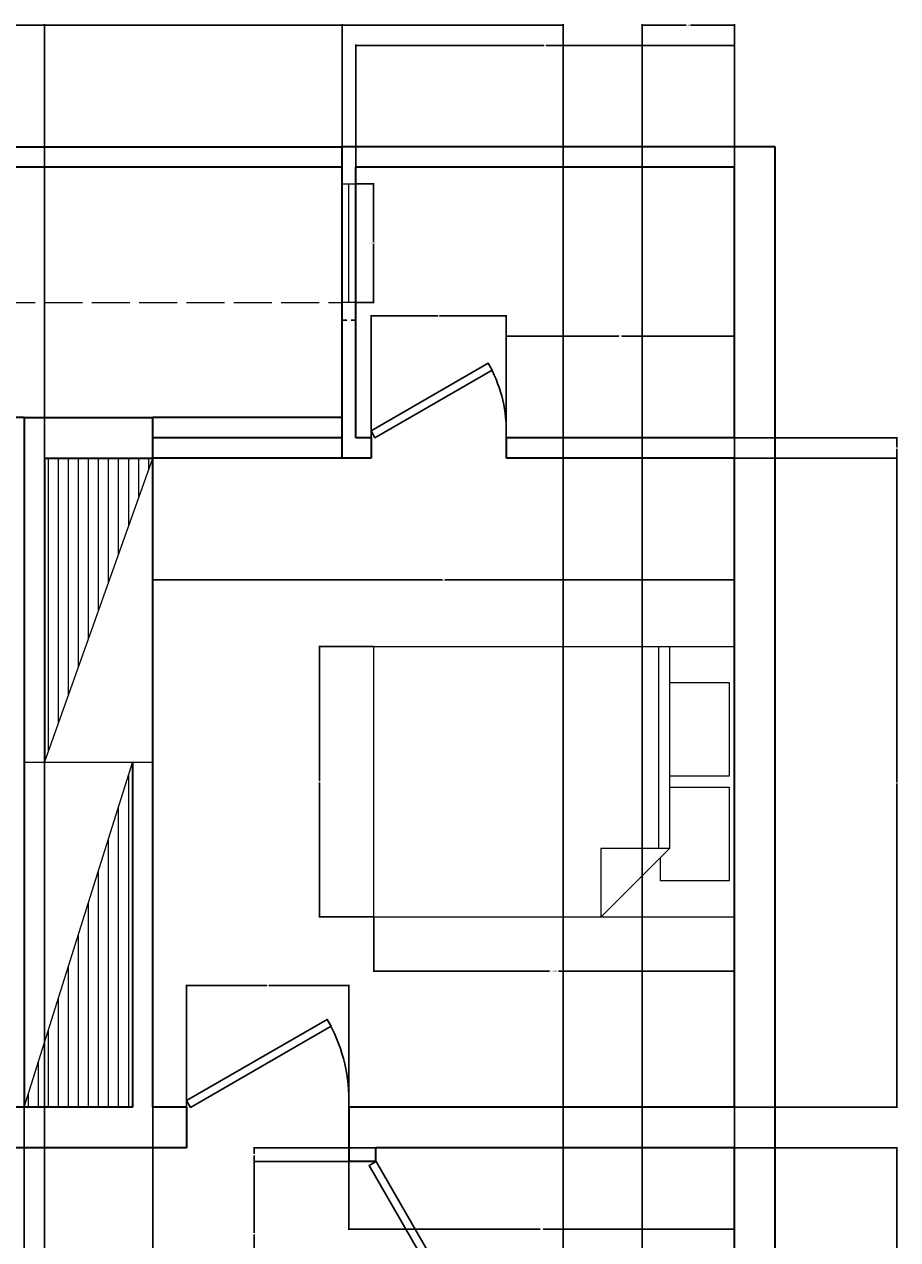
# Model space of a CAD drawing. Units: inches. Extents: x 2599 to 2953, y 557 to 1152.
# Tile 7 of 7: x 2759 to 2953, y 882 to 1152. Entities that reach past the tile are written whole.
import ezdxf

# ---------------------------------------------------------------- set-up
doc = ezdxf.new("R2010")
doc.units = ezdxf.units.IN
doc.linetypes.add('ACAD_ISO02W100', pattern=[15, 12, -3])
for name, color, linetype, lineweight in [('A-ANNO-DIMS', 2, 'Continuous', 18), ('A-DOOR', 4, 'Continuous', 25), ('A-FLOR-CABN', 9, 'Continuous', 18), ('A-FLOR-PATT', 252, 'Continuous', 13), ('A-FURN', 8, 'Continuous', 18), ('A-GLAZ', 4, 'Continuous', 18), ('A-WALL', 7, 'Continuous', 35), ('A-WALL-OVHD', 8, 'ACAD_ISO02W100', 18)]:
    doc.layers.add(name, color=color, linetype=linetype, lineweight=lineweight)
doc.styles.get("Standard").update_dxf_attribs({"font": 'arial.ttf'})
doc.dimstyles.get("Standard").update_dxf_attribs({"dimtxt": 0.18, "dimasz": 0.18, "dimexe": 0.18, "dimexo": 0.0625, "dimgap": 0.09, "dimtad": 0, "dimtih": 1, "dimtoh": 1, "dimdec": 4, "dimzin": 0, "dimdsep": 46, "dimtxsty": 'Standard', "dimcen": 0.09, "dimadec": 0, "dimazin": 0, "dimtfac": 1, "dimtdec": 4, "dimtofl": 0, "dimtmove": 0, "dimatfit": 3, "dimfxl": 1, "dimtolj": 1, "dimtzin": 0, "dimarcsym": 0})

# ---------------------------------------------------------------- blocks, each defined once
blk = doc.blocks.new('*U4')
for p, q in [((0, 0), (0, -6)), ((36, 0), (36, -6))]:
    blk.add_line(p, q)
blk.add_lwpolyline([(0, 0), (31.18, 18), (32.05, 16.48), (0.87, -1.52)], close=True)
blk.add_arc((0, 0), 36, 0, 30)
blk = doc.blocks.new('*U5')
for p, q in [((0, 0), (0, -6)), ((30, 0), (30, -6))]:
    blk.add_line(p, q)
blk.add_lwpolyline([(0, 0), (25.98, 15), (26.86, 13.48), (0.87, -1.52)], close=True)
blk.add_arc((0, 0), 30, 0, 30)
blk = doc.blocks.new('*U6')
for p, q in [((0, 0), (0, -6)), ((32, 0), (32, -6))]:
    blk.add_line(p, q)
blk.add_lwpolyline([(0, 0), (27.71, 16), (28.59, 14.48), (0.87, -1.52)], close=True)
blk.add_arc((0, 0), 32, 0, 30)
blk = doc.blocks.new('Bed - Queen')
for p, q in [((0, -80.00003), (0, 0)), ((0, 0), (59.99999, 0)), ((59.99999, 0), (59.99999, -80.00003)), ((7.99999, -1.2), (28.79998, -1.2)), ((7.99999, -14.4), (7.99999, -1.2)), ((28.79998, -1.2), (28.79998, -14.4)), ((31.19999, -1.2), (51.99999, -1.2)), ((31.19999, -14.4), (31.19999, -1.2)), ((51.99999, -1.2), (51.99999, -16.4)), ((0, -14.4), (44.8, -14.4)), ((59.99999, -29.6), (44.8, -14.4)), ((44.8, -14.4), (44.8, -29.6)), ((44.8, -16.8), (0, -16.8)), ((51.99999, -16.4), (46.79936, -16.4)), ((44.8, -29.6), (59.99999, -29.6)), ((59.99999, -80.00003), (0, -80.00003))]:
    blk.add_line(p, q)
blk = doc.blocks.new('WIN-26_335IN')
for p, q in [((0, 26.33), (3, 26.33)), ((1.5, 0), (1.5, 26.33)), ((3, 0), (0, 0))]:
    blk.add_line(p, q)
blk = doc.blocks.new('*D13')
at = {"layer": 'A-ANNO-DIMS', "color": 0, "lineweight": -2, "transparency": 16777216}
for p, q in [((2832.98, 1116.18), (2837.05, 1116.18)), ((2836.87, 1116), (2836.87, 1103.19)), ((2836.87, 1090.02), (2836.87, 1102.83)), ((2832.98, 1089.84), (2837.05, 1089.84))]:
    blk.add_line(p, q, dxfattribs=at)
at = {"layer": 'A-ANNO-DIMS', "color": 0, "transparency": 16777216}
for points in [[(2836.84, 1116), (2836.9, 1116), (2836.87, 1116.18)], [(2836.84, 1090.02), (2836.9, 1090.02), (2836.87, 1089.84)]]:
    blk.add_solid(points, dxfattribs=at)
at = {"layer": 'Defpoints', "color": 0, "transparency": 16777216}
for p in [(2832.92, 1116.18), (2836.87, 1116.18), (2832.92, 1089.84)]:
    blk.add_point(p, dxfattribs=at)
at = {"layer": 'A-ANNO-DIMS', "color": 0, "transparency": 16777216, "insert": (2836.87, 1103.01), "char_height": 0.18, "attachment_point": 5}
blk.add_mtext('\\A1;WINDOW 26 TYP.', dxfattribs=at)
blk = doc.blocks.new('*D14')
at = {"layer": 'A-ANNO-DIMS', "color": 0, "lineweight": -2, "transparency": 16777216}
for p, q in [((2829.92, 1089.78), (2829.92, 1085.71)), ((2832.92, 1089.78), (2832.92, 1085.71)), ((2830.1, 1085.89), (2830.96, 1085.89)), ((2832.74, 1085.89), (2831.88, 1085.89))]:
    blk.add_line(p, q, dxfattribs=at)
at = {"layer": 'A-ANNO-DIMS', "color": 0, "transparency": 16777216}
for points in [[(2830.1, 1085.92), (2830.1, 1085.86), (2829.92, 1085.89)], [(2832.74, 1085.92), (2832.74, 1085.86), (2832.92, 1085.89)]]:
    blk.add_solid(points, dxfattribs=at)
at = {"layer": 'Defpoints', "color": 0, "transparency": 16777216}
for p in [(2829.92, 1089.84), (2832.92, 1089.84), (2832.92, 1085.89)]:
    blk.add_point(p, dxfattribs=at)
at = {"layer": 'A-ANNO-DIMS', "color": 0, "transparency": 16777216, "insert": (2831.42, 1085.89), "char_height": 0.18, "attachment_point": 5}
blk.add_mtext('\\A1;3 TYP.', dxfattribs=at)
blk = doc.blocks.new('*D15')
at = {"layer": 'A-ANNO-DIMS', "color": 0, "lineweight": -2, "transparency": 16777216}
for p, q in [((2836.92, 953.48), (2836.92, 941.37)), ((2916.92, 953.48), (2916.92, 941.37)), ((2837.1, 941.55), (2875.93, 941.55)), ((2916.74, 941.55), (2877.92, 941.55))]:
    blk.add_line(p, q, dxfattribs=at)
at = {"layer": 'A-ANNO-DIMS', "color": 0, "transparency": 16777216}
for points in [[(2837.1, 941.58), (2837.1, 941.52), (2836.92, 941.55)], [(2916.74, 941.58), (2916.74, 941.52), (2916.92, 941.55)]]:
    blk.add_solid(points, dxfattribs=at)
at = {"layer": 'Defpoints', "color": 0, "transparency": 16777216}
for p in [(2836.92, 953.55), (2916.92, 953.55), (2916.92, 941.55)]:
    blk.add_point(p, dxfattribs=at)
at = {"layer": 'A-ANNO-DIMS', "color": 0, "transparency": 16777216, "insert": (2876.92, 941.55), "char_height": 0.18, "attachment_point": 5}
blk.add_mtext('\\A1;QUEEN BED 80', dxfattribs=at)
blk = doc.blocks.new('*D16')
at = {"layer": 'A-ANNO-DIMS', "color": 0, "lineweight": -2, "transparency": 16777216}
for p, q in [((2836.86, 1013.55), (2824.74, 1013.55)), ((2824.92, 1013.37), (2824.92, 983.73)), ((2824.92, 953.73), (2824.92, 983.36)), ((2836.86, 953.55), (2824.74, 953.55))]:
    blk.add_line(p, q, dxfattribs=at)
at = {"layer": 'A-ANNO-DIMS', "color": 0, "transparency": 16777216}
for points in [[(2824.89, 1013.37), (2824.95, 1013.37), (2824.92, 1013.55)], [(2824.89, 953.73), (2824.95, 953.73), (2824.92, 953.55)]]:
    blk.add_solid(points, dxfattribs=at)
at = {"layer": 'Defpoints', "color": 0, "transparency": 16777216}
for p in [(2836.92, 1013.55), (2824.92, 953.55), (2836.92, 953.55)]:
    blk.add_point(p, dxfattribs=at)
at = {"layer": 'A-ANNO-DIMS', "color": 0, "transparency": 16777216, "insert": (2824.92, 983.55), "char_height": 0.18, "attachment_point": 5}
blk.add_mtext('\\A1;60', dxfattribs=at)
blk = doc.blocks.new('*D21')
at = {"layer": 'A-ANNO-DIMS', "color": 0, "lineweight": -2, "transparency": 16777216}
for p, q in [((2625.92, 1124.28), (2625.92, 557.16)), ((2925.92, 584.28), (2925.92, 557.16)), ((2626.1, 557.34), (2775.63, 557.34)), ((2925.74, 557.34), (2776.21, 557.34))]:
    blk.add_line(p, q, dxfattribs=at)
at = {"layer": 'A-ANNO-DIMS', "color": 0, "transparency": 16777216}
for points in [[(2626.1, 557.37), (2626.1, 557.31), (2625.92, 557.34)], [(2925.74, 557.37), (2925.74, 557.31), (2925.92, 557.34)]]:
    blk.add_solid(points, dxfattribs=at)
at = {"layer": 'Defpoints', "color": 0, "transparency": 16777216}
for p in [(2625.92, 1124.34), (2925.92, 584.34), (2925.92, 557.34)]:
    blk.add_point(p, dxfattribs=at)
at = {"layer": 'A-ANNO-DIMS', "color": 0, "transparency": 16777216, "insert": (2775.92, 557.34), "char_height": 0.18, "attachment_point": 5}
blk.add_mtext('\\A1;300', dxfattribs=at)
blk = doc.blocks.new('*D25')
at = {"layer": 'A-ANNO-DIMS', "color": 0, "lineweight": -2, "transparency": 16777216}
for p, q in [((2916.98, 902.34), (2953.1, 902.34)), ((2952.92, 902.16), (2952.92, 836.52)), ((2952.92, 770.52), (2952.92, 836.16)), ((2916.98, 770.34), (2953.1, 770.34))]:
    blk.add_line(p, q, dxfattribs=at)
at = {"layer": 'A-ANNO-DIMS', "color": 0, "transparency": 16777216}
for points in [[(2952.89, 902.16), (2952.95, 902.16), (2952.92, 902.34)], [(2952.89, 770.52), (2952.95, 770.52), (2952.92, 770.34)]]:
    blk.add_solid(points, dxfattribs=at)
at = {"layer": 'Defpoints', "color": 0, "transparency": 16777216}
for p in [(2916.92, 902.34), (2952.92, 902.34), (2916.92, 770.34)]:
    blk.add_point(p, dxfattribs=at)
at = {"layer": 'A-ANNO-DIMS', "color": 0, "transparency": 16777216, "insert": (2952.92, 836.34), "char_height": 0.18, "attachment_point": 5}
blk.add_mtext('\\A1;132', dxfattribs=at)
blk = doc.blocks.new('*D26')
at = {"layer": 'A-ANNO-DIMS', "color": 0, "lineweight": -2, "transparency": 16777216}
for p, q in [((2837.36, 899.34), (2810.24, 899.34)), ((2810.42, 899.16), (2810.42, 883.52)), ((2810.42, 867.52), (2810.42, 883.16)), ((2837.36, 867.34), (2810.24, 867.34))]:
    blk.add_line(p, q, dxfattribs=at)
at = {"layer": 'A-ANNO-DIMS', "color": 0, "transparency": 16777216}
for points in [[(2810.39, 899.16), (2810.45, 899.16), (2810.42, 899.34)], [(2810.39, 867.52), (2810.45, 867.52), (2810.42, 867.34)]]:
    blk.add_solid(points, dxfattribs=at)
at = {"layer": 'Defpoints', "color": 0, "transparency": 16777216}
for p in [(2810.42, 899.34), (2837.42, 899.34), (2837.42, 867.34)]:
    blk.add_point(p, dxfattribs=at)
at = {"layer": 'A-ANNO-DIMS', "color": 0, "transparency": 16777216, "insert": (2810.42, 883.34), "char_height": 0.18, "attachment_point": 5}
blk.add_mtext('\\A1;32', dxfattribs=at)
blk = doc.blocks.new('*D27')
at = {"layer": 'A-ANNO-DIMS', "color": 0, "lineweight": -2, "transparency": 16777216}
for p, q in [((2837.36, 902.34), (2810.24, 902.34)), ((2810.42, 902.16), (2810.42, 901.02)), ((2810.42, 899.52), (2810.42, 900.66)), ((2837.36, 899.34), (2810.24, 899.34))]:
    blk.add_line(p, q, dxfattribs=at)
at = {"layer": 'A-ANNO-DIMS', "color": 0, "transparency": 16777216}
for points in [[(2810.39, 902.16), (2810.45, 902.16), (2810.42, 902.34)], [(2810.39, 899.52), (2810.45, 899.52), (2810.42, 899.34)]]:
    blk.add_solid(points, dxfattribs=at)
at = {"layer": 'Defpoints', "color": 0, "transparency": 16777216}
for p in [(2810.42, 902.34), (2837.42, 902.34), (2837.42, 899.34)]:
    blk.add_point(p, dxfattribs=at)
at = {"layer": 'A-ANNO-DIMS', "color": 0, "transparency": 16777216, "insert": (2810.42, 900.84), "char_height": 0.18, "attachment_point": 5}
blk.add_mtext('\\A1;3', dxfattribs=at)
blk = doc.blocks.new('*D38')
at = {"layer": 'A-ANNO-DIMS', "color": 0, "lineweight": -2, "transparency": 16777216}
for p, q in [((2763.92, 761.4), (2763.92, 1151.53)), ((2764.1, 1151.35), (2821.14, 1151.35)), ((2878.74, 1151.35), (2821.7, 1151.35)), ((2878.92, 761.4), (2878.92, 1151.53))]:
    blk.add_line(p, q, dxfattribs=at)
at = {"layer": 'A-ANNO-DIMS', "color": 0, "transparency": 16777216}
for points in [[(2764.1, 1151.38), (2764.1, 1151.32), (2763.92, 1151.35)], [(2878.74, 1151.38), (2878.74, 1151.32), (2878.92, 1151.35)]]:
    blk.add_solid(points, dxfattribs=at)
at = {"layer": 'Defpoints', "color": 0, "transparency": 16777216}
for p in [(2878.92, 1151.35), (2763.92, 761.34), (2878.92, 761.34)]:
    blk.add_point(p, dxfattribs=at)
at = {"layer": 'A-ANNO-DIMS', "color": 0, "transparency": 16777216, "insert": (2821.42, 1151.35), "char_height": 0.18, "attachment_point": 5}
blk.add_mtext('\\A1;115', dxfattribs=at)
blk = doc.blocks.new('*D39')
at = {"layer": 'A-ANNO-DIMS', "color": 0, "lineweight": -2, "transparency": 16777216}
for p, q in [((2896.44, 761.4), (2896.44, 1151.53)), ((2896.62, 1151.35), (2906.21, 1151.35)), ((2916.74, 1151.35), (2907.14, 1151.35)), ((2916.92, 761.4), (2916.92, 1151.53))]:
    blk.add_line(p, q, dxfattribs=at)
at = {"layer": 'A-ANNO-DIMS', "color": 0, "transparency": 16777216}
for points in [[(2896.62, 1151.38), (2896.62, 1151.32), (2896.44, 1151.35)], [(2916.74, 1151.38), (2916.74, 1151.32), (2916.92, 1151.35)]]:
    blk.add_solid(points, dxfattribs=at)
at = {"layer": 'Defpoints', "color": 0, "transparency": 16777216}
for p in [(2916.92, 1151.35), (2896.44, 761.34), (2916.92, 761.34)]:
    blk.add_point(p, dxfattribs=at)
at = {"layer": 'A-ANNO-DIMS', "color": 0, "transparency": 16777216, "insert": (2906.68, 1151.35), "char_height": 0.18, "attachment_point": 5}
blk.add_mtext('\\A1;20.483', dxfattribs=at)
blk = doc.blocks.new('*D55')
at = {"layer": 'A-ANNO-DIMS', "color": 0, "lineweight": -2, "transparency": 16777216}
for p, q in [((2759.42, 911.28), (2759.42, 557.16)), ((2787.92, 911.28), (2787.92, 557.16)), ((2759.6, 557.34), (2773.35, 557.34)), ((2787.74, 557.34), (2774, 557.34))]:
    blk.add_line(p, q, dxfattribs=at)
at = {"layer": 'A-ANNO-DIMS', "color": 0, "transparency": 16777216}
for points in [[(2759.6, 557.37), (2759.6, 557.31), (2759.42, 557.34)], [(2787.74, 557.37), (2787.74, 557.31), (2787.92, 557.34)]]:
    blk.add_solid(points, dxfattribs=at)
at = {"layer": 'Defpoints', "color": 0, "transparency": 16777216}
for p in [(2759.42, 911.34), (2787.92, 911.34), (2787.92, 557.34)]:
    blk.add_point(p, dxfattribs=at)
at = {"layer": 'A-ANNO-DIMS', "color": 0, "transparency": 16777216, "insert": (2773.67, 557.34), "char_height": 0.18, "attachment_point": 5}
blk.add_mtext('\\A1;28.5', dxfattribs=at)
blk = doc.blocks.new('*D56')
at = {"layer": 'A-ANNO-DIMS', "color": 0, "lineweight": -2, "transparency": 16777216}
for p, q in [((2787.92, 1055.28), (2787.92, 1028.16)), ((2916.92, 1055.28), (2916.92, 1028.16)), ((2788.1, 1028.34), (2852.14, 1028.34)), ((2916.74, 1028.34), (2852.7, 1028.34))]:
    blk.add_line(p, q, dxfattribs=at)
at = {"layer": 'A-ANNO-DIMS', "color": 0, "transparency": 16777216}
for points in [[(2788.1, 1028.37), (2788.1, 1028.31), (2787.92, 1028.34)], [(2916.74, 1028.37), (2916.74, 1028.31), (2916.92, 1028.34)]]:
    blk.add_solid(points, dxfattribs=at)
at = {"layer": 'Defpoints', "color": 0, "transparency": 16777216}
for p in [(2787.92, 1055.34), (2916.92, 1055.34), (2787.92, 1028.34)]:
    blk.add_point(p, dxfattribs=at)
at = {"layer": 'A-ANNO-DIMS', "color": 0, "transparency": 16777216, "insert": (2852.42, 1028.34), "char_height": 0.18, "attachment_point": 5}
blk.add_mtext('\\A1;129', dxfattribs=at)
blk = doc.blocks.new('*D57')
at = {"layer": 'A-ANNO-DIMS', "color": 0, "lineweight": -2, "transparency": 16777216}
for p, q in [((2916.98, 1055.34), (2953.1, 1055.34)), ((2952.92, 1055.16), (2952.92, 983.52)), ((2952.92, 911.52), (2952.92, 983.16)), ((2916.98, 911.34), (2953.1, 911.34))]:
    blk.add_line(p, q, dxfattribs=at)
at = {"layer": 'A-ANNO-DIMS', "color": 0, "transparency": 16777216}
for points in [[(2952.89, 1055.16), (2952.95, 1055.16), (2952.92, 1055.34)], [(2952.89, 911.52), (2952.95, 911.52), (2952.92, 911.34)]]:
    blk.add_solid(points, dxfattribs=at)
at = {"layer": 'Defpoints', "color": 0, "transparency": 16777216}
for p in [(2916.92, 1055.34), (2952.92, 1055.34), (2916.92, 911.34)]:
    blk.add_point(p, dxfattribs=at)
at = {"layer": 'A-ANNO-DIMS', "color": 0, "transparency": 16777216, "insert": (2952.92, 983.34), "char_height": 0.18, "attachment_point": 5}
blk.add_mtext('\\A1;144', dxfattribs=at)
blk = doc.blocks.new('*D59')
at = {"layer": 'A-ANNO-DIMS', "color": 0, "lineweight": -2, "transparency": 16777216}
for p, q in [((2721.92, 1124.4), (2721.92, 1151.53)), ((2722.1, 1151.35), (2775.64, 1151.35)), ((2829.74, 1151.35), (2776.2, 1151.35)), ((2829.92, 1124.4), (2829.92, 1151.53))]:
    blk.add_line(p, q, dxfattribs=at)
at = {"layer": 'A-ANNO-DIMS', "color": 0, "transparency": 16777216}
for points in [[(2722.1, 1151.38), (2722.1, 1151.32), (2721.92, 1151.35)], [(2829.74, 1151.38), (2829.74, 1151.32), (2829.92, 1151.35)]]:
    blk.add_solid(points, dxfattribs=at)
at = {"layer": 'Defpoints', "color": 0, "transparency": 16777216}
for p in [(2829.92, 1151.35), (2721.92, 1124.34), (2829.92, 1124.34)]:
    blk.add_point(p, dxfattribs=at)
at = {"layer": 'A-ANNO-DIMS', "color": 0, "transparency": 16777216, "insert": (2775.92, 1151.35), "char_height": 0.18, "attachment_point": 5}
blk.add_mtext('\\A1;108', dxfattribs=at)
blk = doc.blocks.new('*D60')
at = {"layer": 'A-ANNO-DIMS', "color": 0, "lineweight": -2, "transparency": 16777216}
for p, q in [((2832.92, 1119.9), (2832.92, 1147.03)), ((2833.1, 1146.85), (2874.7, 1146.85)), ((2916.74, 1146.85), (2875.14, 1146.85)), ((2916.92, 1119.9), (2916.92, 1147.03))]:
    blk.add_line(p, q, dxfattribs=at)
at = {"layer": 'A-ANNO-DIMS', "color": 0, "transparency": 16777216}
for points in [[(2833.1, 1146.88), (2833.1, 1146.82), (2832.92, 1146.85)], [(2916.74, 1146.88), (2916.74, 1146.82), (2916.92, 1146.85)]]:
    blk.add_solid(points, dxfattribs=at)
at = {"layer": 'Defpoints', "color": 0, "transparency": 16777216}
for p in [(2916.92, 1146.85), (2832.92, 1119.84), (2916.92, 1119.84)]:
    blk.add_point(p, dxfattribs=at)
at = {"layer": 'A-ANNO-DIMS', "color": 0, "transparency": 16777216, "insert": (2874.92, 1146.85), "char_height": 0.18, "attachment_point": 5}
blk.add_mtext('\\A1;84', dxfattribs=at)
blk = doc.blocks.new('*D64')
at = {"layer": 'A-ANNO-DIMS', "color": 0, "lineweight": -2, "transparency": 16777216}
for p, q in [((2836.32, 1059.9), (2836.32, 1087.03)), ((2836.5, 1086.85), (2851.1, 1086.85)), ((2866.14, 1086.85), (2851.54, 1086.85)), ((2866.32, 1059.9), (2866.32, 1087.03))]:
    blk.add_line(p, q, dxfattribs=at)
at = {"layer": 'A-ANNO-DIMS', "color": 0, "transparency": 16777216}
for points in [[(2836.5, 1086.88), (2836.5, 1086.82), (2836.32, 1086.85)], [(2866.14, 1086.88), (2866.14, 1086.82), (2866.32, 1086.85)]]:
    blk.add_solid(points, dxfattribs=at)
at = {"layer": 'Defpoints', "color": 0, "transparency": 16777216}
for p in [(2866.32, 1086.85), (2836.32, 1059.84), (2866.32, 1059.84)]:
    blk.add_point(p, dxfattribs=at)
at = {"layer": 'A-ANNO-DIMS', "color": 0, "transparency": 16777216, "insert": (2851.32, 1086.85), "char_height": 0.18, "attachment_point": 5}
blk.add_mtext('\\A1;30', dxfattribs=at)
blk = doc.blocks.new('*D65')
at = {"layer": 'A-ANNO-DIMS', "color": 0, "lineweight": -2, "transparency": 16777216}
for p, q in [((2866.32, 1055.4), (2866.32, 1082.53)), ((2866.5, 1082.35), (2891.3, 1082.35)), ((2916.74, 1082.35), (2891.94, 1082.35)), ((2916.92, 1055.4), (2916.92, 1082.53))]:
    blk.add_line(p, q, dxfattribs=at)
at = {"layer": 'A-ANNO-DIMS', "color": 0, "transparency": 16777216}
for points in [[(2866.5, 1082.38), (2866.5, 1082.32), (2866.32, 1082.35)], [(2916.74, 1082.38), (2916.74, 1082.32), (2916.92, 1082.35)]]:
    blk.add_solid(points, dxfattribs=at)
at = {"layer": 'Defpoints', "color": 0, "transparency": 16777216}
for p in [(2916.92, 1082.35), (2866.32, 1055.34), (2916.92, 1055.34)]:
    blk.add_point(p, dxfattribs=at)
at = {"layer": 'A-ANNO-DIMS', "color": 0, "transparency": 16777216, "insert": (2891.62, 1082.35), "char_height": 0.18, "attachment_point": 5}
blk.add_mtext('\\A1;50.6', dxfattribs=at)
blk = doc.blocks.new('*D68')
at = {"layer": 'A-ANNO-DIMS', "color": 0, "lineweight": -2, "transparency": 16777216}
for p, q in [((2795.42, 911.4), (2795.42, 938.53)), ((2795.6, 938.35), (2813.21, 938.35)), ((2831.24, 938.35), (2813.64, 938.35)), ((2831.42, 911.4), (2831.42, 938.53))]:
    blk.add_line(p, q, dxfattribs=at)
at = {"layer": 'A-ANNO-DIMS', "color": 0, "transparency": 16777216}
for points in [[(2795.6, 938.38), (2795.6, 938.32), (2795.42, 938.35)], [(2831.24, 938.38), (2831.24, 938.32), (2831.42, 938.35)]]:
    blk.add_solid(points, dxfattribs=at)
at = {"layer": 'Defpoints', "color": 0, "transparency": 16777216}
for p in [(2831.42, 938.35), (2795.42, 911.34), (2831.42, 911.34)]:
    blk.add_point(p, dxfattribs=at)
at = {"layer": 'A-ANNO-DIMS', "color": 0, "transparency": 16777216, "insert": (2813.42, 938.35), "char_height": 0.18, "attachment_point": 5}
blk.add_mtext('\\A1;36', dxfattribs=at)
blk = doc.blocks.new('*D69')
at = {"layer": 'A-ANNO-DIMS', "color": 0, "lineweight": -2, "transparency": 16777216}
for p, q in [((2831.42, 911.28), (2831.42, 884.16)), ((2916.92, 911.28), (2916.92, 884.16)), ((2831.6, 884.34), (2873.85, 884.34)), ((2916.74, 884.34), (2874.5, 884.34))]:
    blk.add_line(p, q, dxfattribs=at)
at = {"layer": 'A-ANNO-DIMS', "color": 0, "transparency": 16777216}
for points in [[(2831.6, 884.37), (2831.6, 884.31), (2831.42, 884.34)], [(2916.74, 884.37), (2916.74, 884.31), (2916.92, 884.34)]]:
    blk.add_solid(points, dxfattribs=at)
at = {"layer": 'Defpoints', "color": 0, "transparency": 16777216}
for p in [(2831.42, 911.34), (2916.92, 911.34), (2831.42, 884.34)]:
    blk.add_point(p, dxfattribs=at)
at = {"layer": 'A-ANNO-DIMS', "color": 0, "transparency": 16777216, "insert": (2874.17, 884.34), "char_height": 0.18, "attachment_point": 5}
blk.add_mtext('\\A1;85.5', dxfattribs=at)
blk = doc.blocks.new('*D71')
at = {"layer": 'A-ANNO-DIMS', "color": 0, "lineweight": -2, "transparency": 16777216}
for p, q in [((2829.86, 1119.84), (2598.74, 1119.84)), ((2598.92, 1119.66), (2598.92, 1092.27)), ((2598.92, 1064.52), (2598.92, 1091.91)), ((2787.86, 1064.34), (2598.74, 1064.34))]:
    blk.add_line(p, q, dxfattribs=at)
at = {"layer": 'A-ANNO-DIMS', "color": 0, "transparency": 16777216}
for points in [[(2598.89, 1119.66), (2598.95, 1119.66), (2598.92, 1119.84)], [(2598.89, 1064.52), (2598.95, 1064.52), (2598.92, 1064.34)]]:
    blk.add_solid(points, dxfattribs=at)
at = {"layer": 'Defpoints', "color": 0, "transparency": 16777216}
for p in [(2598.92, 1119.84), (2829.92, 1119.84), (2787.92, 1064.34)]:
    blk.add_point(p, dxfattribs=at)
at = {"layer": 'A-ANNO-DIMS', "color": 0, "transparency": 16777216, "insert": (2598.92, 1092.09), "char_height": 0.18, "attachment_point": 5}
blk.add_mtext('\\A1;55.5', dxfattribs=at)
blk = doc.blocks.new('*D73')
at = {"layer": 'A-ANNO-DIMS', "color": 0, "lineweight": -2, "transparency": 16777216}
for p, q in [((2916.98, 1059.84), (2953.1, 1059.84)), ((2952.92, 1059.66), (2952.92, 1057.77)), ((2952.92, 1055.52), (2952.92, 1057.41)), ((2916.98, 1055.34), (2953.1, 1055.34))]:
    blk.add_line(p, q, dxfattribs=at)
at = {"layer": 'A-ANNO-DIMS', "color": 0, "transparency": 16777216}
for points in [[(2952.89, 1059.66), (2952.95, 1059.66), (2952.92, 1059.84)], [(2952.89, 1055.52), (2952.95, 1055.52), (2952.92, 1055.34)]]:
    blk.add_solid(points, dxfattribs=at)
at = {"layer": 'Defpoints', "color": 0, "transparency": 16777216}
for p in [(2916.92, 1059.84), (2952.92, 1059.84), (2916.92, 1055.34)]:
    blk.add_point(p, dxfattribs=at)
at = {"layer": 'A-ANNO-DIMS', "color": 0, "transparency": 16777216, "insert": (2952.92, 1057.59), "char_height": 0.18, "attachment_point": 5}
blk.add_mtext('\\A1;4.5', dxfattribs=at)

msp = doc.modelspace()

# ---------------------------------------------------------------- hatches: boundary and pattern name
at = {"layer": 'A-FLOR-PATT'}
h = msp.add_hatch(dxfattribs=at)
h.set_pattern_fill('ANSI31', color=256, scale=0.7, angle=45)
h.paths.add_polyline_path([(2763.9211, 987.8417), (2787.9211, 1055.3417), (2763.9211, 1055.3417)])
h.paths.add_polyline_path([(2783.4211, 987.8417), (2759.4211, 911.3417), (2783.4211, 911.3417)])

# ---------------------------------------------------------------- linework, layer by layer
at = {"layer": 'A-FLOR-CABN'}
for p, q in [((2763.9211, 987.8417), (2787.9211, 1055.3417)), ((2787.9211, 987.8417), (2759.4211, 987.8417)), ((2759.4211, 911.3417), (2783.4211, 987.8417))]:
    msp.add_line(p, q, dxfattribs=at)
at = {"layer": 'A-WALL'}
for p, q in [((2721.9211, 1124.3417), (2829.9211, 1124.3417)), ((2925.9211, 1124.3417), (2829.9211, 1124.3417)), ((2829.9211, 1055.3417), (2829.9211, 1124.3417)), ((2925.9211, 584.3417), (2925.9211, 1124.3417)), ((2829.9211, 1119.8417), (2721.9211, 1119.8417)), ((2916.9211, 1119.8417), (2832.9211, 1119.8417)), ((2832.9211, 1059.8417), (2832.9211, 1119.8417)), ((2916.9211, 1059.8417), (2916.9211, 1119.8417)), ((2759.4211, 1064.3417), (2721.9211, 1064.3417)), ((2759.4211, 1064.3417), (2759.4211, 911.3417)), ((2759.4211, 1064.3417), (2787.9211, 1064.3417)), ((2787.9211, 911.3417), (2787.9211, 1064.3417)), ((2829.9211, 1064.3417), (2787.9211, 1064.3417)), ((2829.9211, 1059.8417), (2787.9211, 1059.8417)), ((2836.3211, 1059.8417), (2832.9211, 1059.8417)), ((2836.3211, 1059.8417), (2836.3211, 1055.3417)), ((2916.9211, 1059.8417), (2866.3211, 1059.8417)), ((2866.3211, 1059.8417), (2866.3211, 1055.3417)), ((2763.9211, 1055.3417), (2763.9211, 987.8417)), ((2763.9211, 1055.3417), (2787.9211, 1055.3417)), ((2829.9211, 1055.3417), (2787.9211, 1055.3417)), ((2836.3211, 1055.3417), (2829.9211, 1055.3417)), ((2916.9211, 1055.3417), (2866.3211, 1055.3417)), ((2916.9211, 911.3417), (2916.9211, 1055.3417)), ((2783.4211, 987.8417), (2783.4211, 911.3417)), ((2783.4211, 911.3417), (2753.3499, 911.3417)), ((2795.4243, 911.3417), (2787.9211, 911.3417)), ((2795.4243, 911.3417), (2795.4243, 902.3417)), ((2916.9211, 911.3417), (2831.4243, 911.3417)), ((2831.4243, 911.3417), (2831.4243, 899.3417)), ((2795.4243, 902.3417), (2753.3499, 902.3417)), ((2831.4243, 902.3417), (2831.4211, 902.3417)), ((2916.9211, 902.3417), (2837.4211, 902.3417)), ((2837.4211, 899.3417), (2837.4211, 902.3417)), ((2916.9211, 770.3417), (2916.9211, 902.3417)), ((2837.4211, 899.3417), (2831.4243, 899.3417))]:
    msp.add_line(p, q, dxfattribs=at)
at = {"layer": 'A-WALL-OVHD', "ltscale": 0.7}
msp.add_line((2721.9211, 1089.8417), (2829.9211, 1089.8417), dxfattribs=at)

# ---------------------------------------------------------------- block references
at = {"layer": 'A-DOOR'}
for name, p in [('*U5', (2836.3211, 1061.3417)), ('*U4', (2795.4243, 912.8417))]:
    msp.add_blockref(name, p, dxfattribs=at)
at = {"layer": 'A-DOOR', "rotation": 270}
msp.add_blockref('*U6', (2837.4243, 899.3417), dxfattribs=at)
at = {"layer": 'A-FURN', "rotation": 270}
msp.add_blockref('Bed - Queen', (2916.9211, 1013.5463), dxfattribs=at)
at = {"layer": 'A-GLAZ'}
msp.add_blockref('WIN-26_335IN', (2829.921, 1089.842), dxfattribs=at)

# ---------------------------------------------------------------- dimensions: what is measured, and where the dimension line sits
at = {"layer": 'A-ANNO-DIMS'}
for base, p1, p2, override, picture, middle in [((2829.9211, 1151.3452), (2721.9211, 1124.3417), (2829.9211, 1124.3417), {"dimdec": 0, "dimlfac": 1, "dimrnd": 0, "dimzin": 0, "dimdsep": 46, "dimlunit": 2}, '*D59', (2775.9211, 1151.3452)), ((2878.9211, 1151.3452), (2763.9211, 761.3417), (2878.9211, 761.3417), {"dimdec": 0, "dimlfac": 1, "dimrnd": 0, "dimzin": 0, "dimdsep": 46, "dimlunit": 2}, '*D38', (2821.4211, 1151.3452)), ((2916.92111, 1151.34517), (2896.43762, 761.34167), (2916.92111, 761.34167), {"dimdec": 3, "dimlfac": 1, "dimrnd": 0, "dimzin": 0, "dimdsep": 46, "dimlunit": 2}, '*D39', (2906.67936, 1151.34517)), ((2916.9211, 1146.8452), (2832.9211, 1119.8417), (2916.9211, 1119.8417), {"dimdec": 0, "dimlfac": 1, "dimrnd": 0, "dimzin": 0, "dimdsep": 46, "dimlunit": 2}, '*D60', (2874.9211, 1146.8452)), ((2925.9211, 557.3382), (2625.9211, 1124.3417), (2925.9211, 584.3417), {"dimdec": 0, "dimlfac": 1, "dimrnd": 0, "dimzin": 0, "dimdsep": 46, "dimlunit": 2}, '*D21', (2775.9211, 557.3382)), ((2866.3211, 1086.8452), (2836.3211, 1059.8417), (2866.3211, 1059.8417), {"dimdec": 0, "dimlfac": 1, "dimrnd": 0, "dimzin": 0, "dimdsep": 46, "dimlunit": 2}, '*D64', (2851.3211, 1086.8452)), ((2916.9211, 1082.3452), (2866.3211, 1055.3417), (2916.9211, 1055.3417), {"dimdec": 1, "dimlfac": 1, "dimrnd": 0, "dimzin": 0, "dimdsep": 46, "dimlunit": 2}, '*D65', (2891.6211, 1082.3452)), ((2831.4243, 938.3452), (2795.4243, 911.3417), (2831.4243, 911.3417), {"dimdec": 0, "dimlfac": 1, "dimrnd": 0, "dimzin": 0, "dimdsep": 46, "dimlunit": 2}, '*D68', (2813.4243, 938.3452)), ((2787.9211, 557.3382), (2759.4211, 911.3417), (2787.9211, 911.3417), {"dimdec": 1, "dimlfac": 1, "dimrnd": 0, "dimzin": 0, "dimdsep": 46, "dimlunit": 2}, '*D55', (2773.6711, 557.3382))]:
    dim = msp.add_linear_dim(base=base, p1=p1, p2=p2, dimstyle='Standard', override=override, dxfattribs=at)
    dim.commit()
    dim.dimension.update_dxf_attribs({"geometry": picture, "text_midpoint": middle})
for base, p1, p2, angle, override, picture, middle in [((2598.9176, 1119.8417), (2787.9211, 1064.3417), (2829.9211, 1119.8417), 90, {"dimdec": 1, "dimlfac": 1, "dimrnd": 0, "dimzin": 0, "dimdsep": 46, "dimlunit": 2}, '*D71', (2598.9176, 1092.0917)), ((2952.9246, 1059.8417), (2916.9211, 1055.3417), (2916.9211, 1059.8417), 90, {"dimdec": 1, "dimlfac": 1, "dimrnd": 0, "dimzin": 0, "dimdsep": 46, "dimlunit": 2}, '*D73', (2952.9246, 1057.5917)), ((2787.9211, 1028.3382), (2916.9211, 1055.3417), (2787.9211, 1055.3417), 180, {"dimdec": 0, "dimlfac": 1, "dimrnd": 0, "dimzin": 0, "dimdsep": 46, "dimlunit": 2}, '*D56', (2852.4211, 1028.3382)), ((2952.9246, 1055.3417), (2916.9211, 911.3417), (2916.9211, 1055.3417), 90, {"dimdec": 0, "dimlfac": 1, "dimrnd": 0, "dimzin": 0, "dimdsep": 46, "dimlunit": 2}, '*D57', (2952.9246, 983.3417)), ((2824.9211, 953.5463), (2836.9211, 1013.5463), (2836.9211, 953.5463), 270, {"dimdec": 0, "dimlfac": 1, "dimrnd": 0, "dimzin": 0, "dimdsep": 46, "dimlunit": 2}, '*D16', (2824.9211, 983.5463)), ((2831.4243, 884.3382), (2916.9211, 911.3417), (2831.4243, 911.3417), 180, {"dimdec": 1, "dimlfac": 1, "dimrnd": 0, "dimzin": 0, "dimdsep": 46, "dimlunit": 2}, '*D69', (2874.1727, 884.3382)), ((2810.4176, 902.3417), (2837.4211, 899.3417), (2837.4211, 902.3417), 90, {"dimdec": 0, "dimlfac": 1, "dimrnd": 0, "dimzin": 0, "dimdsep": 46, "dimlunit": 2}, '*D27', (2810.4176, 900.8417)), ((2952.9246, 902.3417), (2916.9211, 770.3417), (2916.9211, 902.3417), 90, {"dimdec": 0, "dimlfac": 1, "dimrnd": 0, "dimzin": 0, "dimdsep": 46, "dimlunit": 2}, '*D25', (2952.9246, 836.3417)), ((2810.4176, 899.3417), (2837.4211, 867.3417), (2837.4211, 899.3417), 90, {"dimdec": 0, "dimlfac": 1, "dimrnd": 0, "dimzin": 0, "dimdsep": 46, "dimlunit": 2}, '*D26', (2810.4176, 883.3417))]:
    dim = msp.add_linear_dim(base=base, p1=p1, p2=p2, angle=angle, dimstyle='Standard', override=override, dxfattribs=at)
    dim.commit()
    dim.dimension.update_dxf_attribs({"geometry": picture, "text_midpoint": middle})
dim = msp.add_linear_dim(base=(2836.8714, 1116.1768), p1=(2832.9211, 1089.8417), p2=(2832.9211, 1116.1768), angle=90, text='WINDOW <> TYP.', dimstyle='Standard', override={"dimdec": 0, "dimlfac": 1, "dimrnd": 0, "dimzin": 0, "dimdsep": 46, "dimlunit": 2}, dxfattribs=at)
dim.commit()
dim.dimension.update_dxf_attribs({"geometry": '*D13', "text_midpoint": (2836.8714, 1103.0092)})
for base, p1, p2, text, picture, middle in [((2832.9211, 1085.8914), (2829.9211, 1089.8417), (2832.9211, 1089.8417), '<> TYP.', '*D14', (2831.4211, 1085.8914)), ((2916.9211, 941.5463), (2836.9211, 953.5463), (2916.9211, 953.5463), 'QUEEN BED <>', '*D15', (2876.9211, 941.5463))]:
    dim = msp.add_linear_dim(base=base, p1=p1, p2=p2, text=text, dimstyle='Standard', override={"dimdec": 0, "dimlfac": 1, "dimrnd": 0, "dimzin": 0, "dimdsep": 46, "dimlunit": 2}, dxfattribs=at)
    dim.commit()
    dim.dimension.update_dxf_attribs({"geometry": picture, "text_midpoint": middle})

doc.saveas('drawing.dxf')
